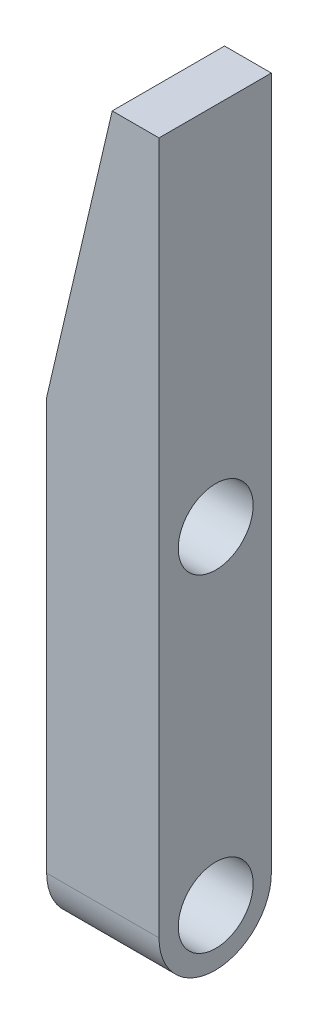
ISO-10303-21;
HEADER;
FILE_DESCRIPTION(('STEP AP214'),'2;1');
FILE_NAME('part.step','',(''),(''),'','','');
FILE_SCHEMA(('AUTOMOTIVE_DESIGN { 1 0 10303 214 1 1 1 1 }'));
ENDSEC;
DATA;
#1=APPLICATION_CONTEXT('core data for automotive mechanical design processes');
#2=APPLICATION_PROTOCOL_DEFINITION('international standard','automotive_design',2000,#1);
#3=PRODUCT_CONTEXT('',#1,'mechanical');
#4=PRODUCT('Part','Part','',(#3));
#5=PRODUCT_RELATED_PRODUCT_CATEGORY('part','',(#4));
#6=PRODUCT_DEFINITION_FORMATION('','',#4);
#7=PRODUCT_DEFINITION_CONTEXT('part definition',#1,'design');
#8=PRODUCT_DEFINITION('design','',#6,#7);
#9=PRODUCT_DEFINITION_SHAPE('','',#8);
#10=(LENGTH_UNIT() NAMED_UNIT(*) SI_UNIT(.MILLI.,.METRE.));
#11=(NAMED_UNIT(*) PLANE_ANGLE_UNIT() SI_UNIT($,.RADIAN.));
#12=(NAMED_UNIT(*) SI_UNIT($,.STERADIAN.) SOLID_ANGLE_UNIT());
#13=UNCERTAINTY_MEASURE_WITH_UNIT(LENGTH_MEASURE(1.E-05),#10,'distance_accuracy_value','');
#14=(GEOMETRIC_REPRESENTATION_CONTEXT(3) GLOBAL_UNCERTAINTY_ASSIGNED_CONTEXT((#13)) GLOBAL_UNIT_ASSIGNED_CONTEXT((#10,
#11,#12)) REPRESENTATION_CONTEXT('',''));
#15=CARTESIAN_POINT('',(0.,0.,0.));
#16=DIRECTION('',(0.,0.,1.));
#17=DIRECTION('',(1.,0.,0.));
#18=AXIS2_PLACEMENT_3D('',#15,#16,#17);
#19=CARTESIAN_POINT('',(0.,-74.,6.));
#20=DIRECTION('',(-1.,0.,0.));
#21=DIRECTION('',(0.,0.,1.));
#22=AXIS2_PLACEMENT_3D('',#19,#20,#21);
#23=PLANE('',#22);
#24=CARTESIAN_POINT('',(0.,-39.,-0.0558484938406878));
#25=DIRECTION('',(1.,0.,0.));
#26=DIRECTION('',(0.,0.,-1.));
#27=AXIS2_PLACEMENT_3D('',#24,#25,#26);
#28=CIRCLE('',#27,3.99999999999999);
#29=CARTESIAN_POINT('',(0.,-39.,-4.05584849384068));
#30=VERTEX_POINT('',#29);
#31=EDGE_CURVE('E166',#30,#30,#28,.T.);
#32=ORIENTED_EDGE('',*,*,#31,.F.);
#33=EDGE_LOOP('',(#32));
#34=FACE_BOUND('',#33,.T.);
#35=DIRECTION('',(0.,1.,0.));
#36=VECTOR('',#35,1.);
#37=CARTESIAN_POINT('',(0.,-74.,6.));
#38=LINE('',#37,#36);
#39=CARTESIAN_POINT('',(0.,-74.,6.));
#40=VERTEX_POINT('',#39);
#41=CARTESIAN_POINT('',(0.,0.,6.));
#42=VERTEX_POINT('',#41);
#43=EDGE_CURVE('E119',#40,#42,#38,.T.);
#44=ORIENTED_EDGE('',*,*,#43,.F.);
#45=CARTESIAN_POINT('',(0.,-74.,0.));
#46=DIRECTION('',(1.,0.,0.));
#47=DIRECTION('',(0.,0.,-1.));
#48=AXIS2_PLACEMENT_3D('',#45,#46,#47);
#49=CIRCLE('',#48,6.);
#50=CARTESIAN_POINT('',(0.,-74.,-6.));
#51=VERTEX_POINT('',#50);
#52=EDGE_CURVE('E121',#40,#51,#49,.T.);
#53=ORIENTED_EDGE('',*,*,#52,.T.);
#54=DIRECTION('',(0.,1.,0.));
#55=VECTOR('',#54,1.);
#56=CARTESIAN_POINT('',(0.,-74.,-6.));
#57=LINE('',#56,#55);
#58=CARTESIAN_POINT('',(0.,0.,-6.));
#59=VERTEX_POINT('',#58);
#60=EDGE_CURVE('E107',#51,#59,#57,.T.);
#61=ORIENTED_EDGE('',*,*,#60,.T.);
#62=DIRECTION('',(0.,0.,-1.));
#63=VECTOR('',#62,1.);
#64=CARTESIAN_POINT('',(0.,0.,6.));
#65=LINE('',#64,#63);
#66=EDGE_CURVE('E11',#42,#59,#65,.T.);
#67=ORIENTED_EDGE('',*,*,#66,.F.);
#68=EDGE_LOOP('',(#44,#53,#61,#67));
#69=FACE_BOUND('',#68,.T.);
#70=CARTESIAN_POINT('',(0.,-74.,-0.0558484938406878));
#71=DIRECTION('',(1.,0.,0.));
#72=DIRECTION('',(0.,0.,-1.));
#73=AXIS2_PLACEMENT_3D('',#70,#71,#72);
#74=CIRCLE('',#73,3.99999999999999);
#75=CARTESIAN_POINT('',(0.,-74.,-4.05584849384068));
#76=VERTEX_POINT('',#75);
#77=EDGE_CURVE('E170',#76,#76,#74,.T.);
#78=ORIENTED_EDGE('',*,*,#77,.F.);
#79=EDGE_LOOP('',(#78));
#80=FACE_BOUND('',#79,.T.);
#81=ADVANCED_FACE('F39',(#34,#69,#80),#23,.F.);
#82=CARTESIAN_POINT('',(0.,0.,6.));
#83=DIRECTION('',(0.,-1.,0.));
#84=DIRECTION('',(0.,0.,-1.));
#85=AXIS2_PLACEMENT_3D('',#82,#83,#84);
#86=PLANE('',#85);
#87=DIRECTION('',(-1.,0.,0.));
#88=VECTOR('',#87,1.);
#89=CARTESIAN_POINT('',(0.,0.,-6.));
#90=LINE('',#89,#88);
#91=CARTESIAN_POINT('',(-5.,0.,-6.));
#92=VERTEX_POINT('',#91);
#93=EDGE_CURVE('E112',#59,#92,#90,.T.);
#94=ORIENTED_EDGE('',*,*,#93,.T.);
#95=DIRECTION('',(0.,0.,-1.));
#96=VECTOR('',#95,1.);
#97=CARTESIAN_POINT('',(-5.,0.,6.));
#98=LINE('',#97,#96);
#99=CARTESIAN_POINT('',(-5.,0.,6.));
#100=VERTEX_POINT('',#99);
#101=EDGE_CURVE('E50',#100,#92,#98,.T.);
#102=ORIENTED_EDGE('',*,*,#101,.F.);
#103=DIRECTION('',(-1.,0.,0.));
#104=VECTOR('',#103,1.);
#105=CARTESIAN_POINT('',(0.,0.,6.));
#106=LINE('',#105,#104);
#107=EDGE_CURVE('E86',#42,#100,#106,.T.);
#108=ORIENTED_EDGE('',*,*,#107,.F.);
#109=ORIENTED_EDGE('',*,*,#66,.T.);
#110=EDGE_LOOP('',(#94,#102,#108,#109));
#111=FACE_BOUND('',#110,.T.);
#112=ADVANCED_FACE('F131',(#111),#86,.F.);
#113=CARTESIAN_POINT('',(-5.,0.,6.));
#114=DIRECTION('',(0.973841209741793,-0.227229615606418,0.));
#115=DIRECTION('',(0.227229615606418,0.973841209741793,0.));
#116=AXIS2_PLACEMENT_3D('',#113,#114,#115);
#117=PLANE('',#116);
#118=DIRECTION('',(-0.227229615606418,-0.973841209741793,0.));
#119=VECTOR('',#118,1.);
#120=CARTESIAN_POINT('',(-5.,0.,-6.));
#121=LINE('',#120,#119);
#122=CARTESIAN_POINT('',(-12.,-30.,-6.));
#123=VERTEX_POINT('',#122);
#124=EDGE_CURVE('E71',#92,#123,#121,.T.);
#125=ORIENTED_EDGE('',*,*,#124,.T.);
#126=DIRECTION('',(0.,0.,-1.));
#127=VECTOR('',#126,1.);
#128=CARTESIAN_POINT('',(-12.,-30.,6.));
#129=LINE('',#128,#127);
#130=CARTESIAN_POINT('',(-12.,-30.,6.));
#131=VERTEX_POINT('',#130);
#132=EDGE_CURVE('E98',#131,#123,#129,.T.);
#133=ORIENTED_EDGE('',*,*,#132,.F.);
#134=DIRECTION('',(-0.227229615606418,-0.973841209741793,0.));
#135=VECTOR('',#134,1.);
#136=CARTESIAN_POINT('',(-5.,0.,6.));
#137=LINE('',#136,#135);
#138=EDGE_CURVE('E91',#100,#131,#137,.T.);
#139=ORIENTED_EDGE('',*,*,#138,.F.);
#140=ORIENTED_EDGE('',*,*,#101,.T.);
#141=EDGE_LOOP('',(#125,#133,#139,#140));
#142=FACE_BOUND('',#141,.T.);
#143=ADVANCED_FACE('F97',(#142),#117,.F.);
#144=CARTESIAN_POINT('',(-12.,-30.,6.));
#145=DIRECTION('',(1.,0.,0.));
#146=DIRECTION('',(0.,1.,0.));
#147=AXIS2_PLACEMENT_3D('',#144,#145,#146);
#148=PLANE('',#147);
#149=CARTESIAN_POINT('',(-12.,-74.,-0.0558484938406878));
#150=DIRECTION('',(1.,0.,0.));
#151=DIRECTION('',(0.,1.,0.));
#152=AXIS2_PLACEMENT_3D('',#149,#150,#151);
#153=CIRCLE('',#152,4.);
#154=CARTESIAN_POINT('',(-12.,-70.,-0.0558484938406878));
#155=VERTEX_POINT('',#154);
#156=EDGE_CURVE('E163',#155,#155,#153,.T.);
#157=ORIENTED_EDGE('',*,*,#156,.T.);
#158=EDGE_LOOP('',(#157));
#159=FACE_BOUND('',#158,.T.);
#160=CARTESIAN_POINT('',(-12.,-39.,-0.0558484938406878));
#161=DIRECTION('',(1.,0.,0.));
#162=DIRECTION('',(0.,1.,0.));
#163=AXIS2_PLACEMENT_3D('',#160,#161,#162);
#164=CIRCLE('',#163,3.99999999999999);
#165=CARTESIAN_POINT('',(-12.,-35.,-0.0558484938406878));
#166=VERTEX_POINT('',#165);
#167=EDGE_CURVE('E130',#166,#166,#164,.T.);
#168=ORIENTED_EDGE('',*,*,#167,.T.);
#169=EDGE_LOOP('',(#168));
#170=FACE_BOUND('',#169,.T.);
#171=DIRECTION('',(0.,-1.,0.));
#172=VECTOR('',#171,1.);
#173=CARTESIAN_POINT('',(-12.,-30.,-6.));
#174=LINE('',#173,#172);
#175=CARTESIAN_POINT('',(-12.,-74.,-6.));
#176=VERTEX_POINT('',#175);
#177=EDGE_CURVE('E78',#123,#176,#174,.T.);
#178=ORIENTED_EDGE('',*,*,#177,.T.);
#179=CARTESIAN_POINT('',(-12.,-74.,0.));
#180=DIRECTION('',(1.,0.,0.));
#181=DIRECTION('',(0.,1.,0.));
#182=AXIS2_PLACEMENT_3D('',#179,#180,#181);
#183=CIRCLE('',#182,6.);
#184=CARTESIAN_POINT('',(-12.,-74.,6.));
#185=VERTEX_POINT('',#184);
#186=EDGE_CURVE('E103',#176,#185,#183,.F.);
#187=ORIENTED_EDGE('',*,*,#186,.T.);
#188=DIRECTION('',(0.,-1.,0.));
#189=VECTOR('',#188,1.);
#190=CARTESIAN_POINT('',(-12.,-30.,6.));
#191=LINE('',#190,#189);
#192=EDGE_CURVE('E96',#131,#185,#191,.T.);
#193=ORIENTED_EDGE('',*,*,#192,.F.);
#194=ORIENTED_EDGE('',*,*,#132,.T.);
#195=EDGE_LOOP('',(#178,#187,#193,#194));
#196=FACE_BOUND('',#195,.T.);
#197=ADVANCED_FACE('F101',(#159,#170,#196),#148,.F.);
#198=CARTESIAN_POINT('',(0.,0.,6.));
#199=DIRECTION('',(0.,0.,1.));
#200=DIRECTION('',(1.,0.,0.));
#201=AXIS2_PLACEMENT_3D('',#198,#199,#200);
#202=PLANE('',#201);
#203=ORIENTED_EDGE('',*,*,#43,.T.);
#204=ORIENTED_EDGE('',*,*,#107,.T.);
#205=ORIENTED_EDGE('',*,*,#138,.T.);
#206=ORIENTED_EDGE('',*,*,#192,.T.);
#207=DIRECTION('',(1.,0.,0.));
#208=VECTOR('',#207,1.);
#209=CARTESIAN_POINT('',(-12.,-74.,6.));
#210=LINE('',#209,#208);
#211=EDGE_CURVE('E54',#185,#40,#210,.T.);
#212=ORIENTED_EDGE('',*,*,#211,.T.);
#213=EDGE_LOOP('',(#203,#204,#205,#206,#212));
#214=FACE_BOUND('',#213,.T.);
#215=ADVANCED_FACE('F94',(#214),#202,.T.);
#216=CARTESIAN_POINT('',(0.,0.,-6.));
#217=DIRECTION('',(0.,0.,1.));
#218=DIRECTION('',(1.,0.,0.));
#219=AXIS2_PLACEMENT_3D('',#216,#217,#218);
#220=PLANE('',#219);
#221=ORIENTED_EDGE('',*,*,#60,.F.);
#222=DIRECTION('',(1.,0.,0.));
#223=VECTOR('',#222,1.);
#224=CARTESIAN_POINT('',(-12.,-74.,-6.));
#225=LINE('',#224,#223);
#226=EDGE_CURVE('E113',#176,#51,#225,.T.);
#227=ORIENTED_EDGE('',*,*,#226,.F.);
#228=ORIENTED_EDGE('',*,*,#177,.F.);
#229=ORIENTED_EDGE('',*,*,#124,.F.);
#230=ORIENTED_EDGE('',*,*,#93,.F.);
#231=EDGE_LOOP('',(#221,#227,#228,#229,#230));
#232=FACE_BOUND('',#231,.T.);
#233=ADVANCED_FACE('F118',(#232),#220,.F.);
#234=CARTESIAN_POINT('',(-28.9705627484771,-74.,0.));
#235=DIRECTION('',(1.,0.,0.));
#236=DIRECTION('',(0.,0.,-1.));
#237=AXIS2_PLACEMENT_3D('',#234,#235,#236);
#238=CYLINDRICAL_SURFACE('',#237,6.);
#239=ORIENTED_EDGE('',*,*,#211,.F.);
#240=ORIENTED_EDGE('',*,*,#186,.F.);
#241=ORIENTED_EDGE('',*,*,#226,.T.);
#242=ORIENTED_EDGE('',*,*,#52,.F.);
#243=EDGE_LOOP('',(#239,#240,#241,#242));
#244=FACE_BOUND('',#243,.T.);
#245=ADVANCED_FACE('F125',(#244),#238,.T.);
#246=CARTESIAN_POINT('',(0.,-39.,-0.0558484938406878));
#247=DIRECTION('',(1.,0.,0.));
#248=DIRECTION('',(0.,0.,-1.));
#249=AXIS2_PLACEMENT_3D('',#246,#247,#248);
#250=CYLINDRICAL_SURFACE('',#249,3.99999999999999);
#251=ORIENTED_EDGE('',*,*,#167,.F.);
#252=EDGE_LOOP('',(#251));
#253=FACE_BOUND('',#252,.T.);
#254=ORIENTED_EDGE('',*,*,#31,.T.);
#255=EDGE_LOOP('',(#254));
#256=FACE_BOUND('',#255,.T.);
#257=ADVANCED_FACE('F155',(#253,#256),#250,.F.);
#258=CARTESIAN_POINT('',(0.,-74.,-0.0558484938406878));
#259=DIRECTION('',(1.,0.,0.));
#260=DIRECTION('',(0.,0.,-1.));
#261=AXIS2_PLACEMENT_3D('',#258,#259,#260);
#262=CYLINDRICAL_SURFACE('',#261,4.);
#263=ORIENTED_EDGE('',*,*,#156,.F.);
#264=EDGE_LOOP('',(#263));
#265=FACE_BOUND('',#264,.T.);
#266=ORIENTED_EDGE('',*,*,#77,.T.);
#267=EDGE_LOOP('',(#266));
#268=FACE_BOUND('',#267,.T.);
#269=ADVANCED_FACE('F154',(#265,#268),#262,.F.);
#270=CLOSED_SHELL('',(#81,#112,#143,#197,#215,#233,#245,#257,#269));
#271=MANIFOLD_SOLID_BREP('B2',#270);
#272=ADVANCED_BREP_SHAPE_REPRESENTATION('',(#18,#271),#14);
#273=SHAPE_DEFINITION_REPRESENTATION(#9,#272);
ENDSEC;
END-ISO-10303-21;
